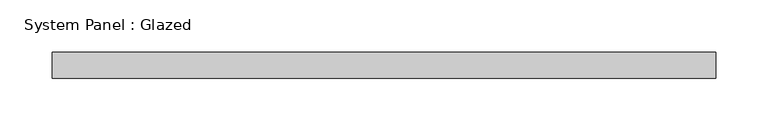
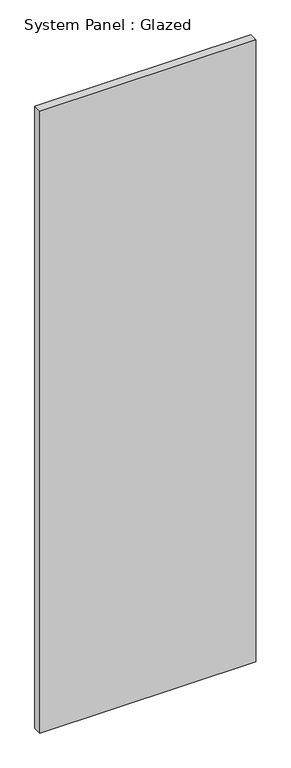
"""IFC4 building model written with IfcOpenShell, lengths in millimetres: plate geometry, System Panel : Glazed."""

from ifc_helpers import new_model, si_unit, origin, origin_with_axes, place, context, project, spatial, polyline, outline, extrude, source, transform, mapped, element, save


def system_panel_glazed_678ad2c6(model_context):
    return source(origin(), model_context, "Body", "SweptSolid", [
        extrude(outline(polyline([(318.6218115, 24.5), (-318.6218115, 24.5), (-318.6218115, 49.5), (318.6218115, 49.5), (318.6218115, 24.5)])), origin_with_axes(), (0.0, 0.0, 1.0), 1938.8741491),
    ])


if __name__ == "__main__":
    model = new_model("IFC4")
    model_context = context("Model", 3, world=origin())
    ifc_project = project(units=[si_unit("LENGTHUNIT", "METRE", prefix="MILLI")], contexts=[model_context])
    site = spatial("IfcSite", under=ifc_project)
    building = spatial("IfcBuilding", under=site)
    placement = place(None, origin())
    system_panel_glazed_shape = system_panel_glazed_678ad2c6(model_context)
    element("IfcPlate", 1, ObjectType="System Panel : Glazed", at=placement, inside=building, context=model_context, shape_type="MappedRepresentation", body=[
        mapped(system_panel_glazed_shape, transform((0.0, 0.0, 0.0), x_axis=(1.0, 0.0, 0.0), y_axis=(0.0, 1.0, 0.0), z_axis=(0.0, 0.0, 1.0))),
    ])
    save(model, "model.ifc")

# Revit data of these elements
# Type "System Panel : Glazed"
#   Keynote = "H11"
#   Construction Type Id = "GSP4R"
#   Analytic Construction = "1/8 in Pilkington single glazing"
#   Visual Light Transmittance = 0.9
#   Solar Heat Gain Coefficient = 0.86
#   Heat Transfer Coefficient (U) = 6.7069 W/(m²·K)
#   Define Thermal Properties by = 1
# Element 1 (IfcPlate, "System Panel : Glazed")
#   Materials on its faces: "Glass"
# Materials
#   "Glass": class "Glass", colour RGB 0 128 192, transparency 0.9, Description = "Soda Lime Glass", Cost = 0
